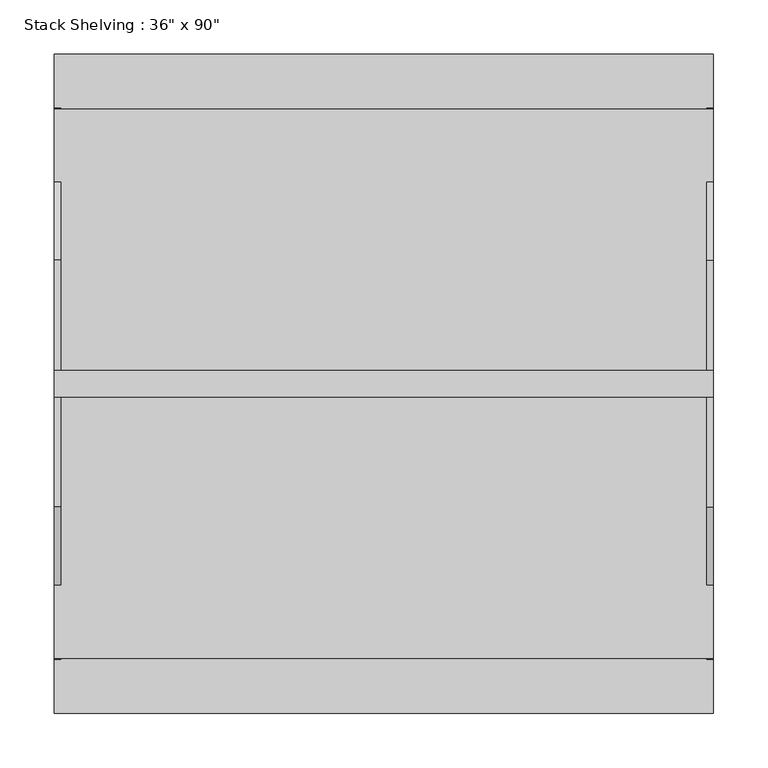
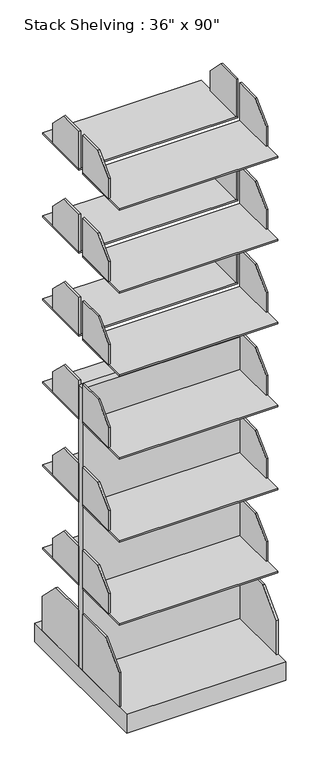
"""IFC4 building model written with IfcOpenShell, lengths in millimetres: proxy geometry."""

from ifc_helpers import new_model, si_unit, frame, origin, origin_with_axes, place, context, project, spatial, polyline, outline, extrude, source, transform, mapped, element, save


def proxy_279d5ef4(model_context):
    return source(origin(), model_context, "Body", "SweptSolid", [
        extrude(outline(polyline([(12.7, 2247.9), (114.3, 2247.9), (186.142049, 2176.057951), (186.142049, 2095.5), (12.7, 2095.5), (12.7, 2247.9)])), frame((-304.8, 0.0, 0.0), z_axis=(1.0, 0.0, 0.0), x_axis=(0.0, 1.0, 0.0)), (0.0, 0.0, 1.0), 6.35),
        extrude(outline(polyline([(165.1, 304.8), (254.9025612, 214.9974388), (254.9025612, 76.2), (12.7, 76.2), (12.7, 304.8), (165.1, 304.8)])), frame((-304.8, 0.0, 0.0), z_axis=(1.0, 0.0, 0.0), x_axis=(0.0, 1.0, 0.0)), (0.0, 0.0, 1.0), 6.35),
        extrude(outline(polyline([(12.7, 1911.35), (114.3, 1911.35), (186.142049, 1839.507951), (186.142049, 1758.95), (12.7, 1758.95), (12.7, 1911.35)])), frame((-304.8, 0.0, 0.0), z_axis=(1.0, 0.0, 0.0), x_axis=(0.0, 1.0, 0.0)), (0.0, 0.0, 1.0), 6.35),
        extrude(outline(polyline([(12.8886472, 1574.8), (114.4886472, 1574.8), (186.3306961, 1502.957951), (186.3306961, 1422.4), (12.8886472, 1422.4), (12.8886472, 1574.8)])), frame((-304.8, 0.0, 0.0), z_axis=(1.0, 0.0, 0.0), x_axis=(0.0, 1.0, 0.0)), (0.0, 0.0, 1.0), 6.35),
        extrude(outline(polyline([(12.8886472, 1238.25), (114.4886472, 1238.25), (186.3306961, 1166.407951), (186.3306961, 1085.85), (12.8886472, 1085.85), (12.8886472, 1238.25)])), frame((-304.8, 0.0, 0.0), z_axis=(1.0, 0.0, 0.0), x_axis=(0.0, 1.0, 0.0)), (0.0, 0.0, 1.0), 6.35),
        extrude(outline(polyline([(12.7, 901.7), (114.3, 901.7), (186.142049, 829.857951), (186.142049, 749.3), (12.7, 749.3), (12.7, 901.7)])), frame((-304.8, 0.0, 0.0), z_axis=(1.0, 0.0, 0.0), x_axis=(0.0, 1.0, 0.0)), (0.0, 0.0, 1.0), 6.35),
        extrude(outline(polyline([(12.7, 565.15), (114.3, 565.15), (186.142049, 493.307951), (186.142049, 412.75), (12.7, 412.75), (12.7, 565.15)])), frame((-304.8, 0.0, 0.0), z_axis=(1.0, 0.0, 0.0), x_axis=(0.0, 1.0, 0.0)), (0.0, 0.0, 1.0), 6.35),
        extrude(outline(polyline([(-12.7, 2247.9), (-12.7, 2095.5), (-186.142049, 2095.5), (-186.142049, 2176.057951), (-114.3, 2247.9), (-12.7, 2247.9)])), frame((-304.8, 0.0, 0.0), z_axis=(1.0, 0.0, 0.0), x_axis=(0.0, 1.0, 0.0)), (0.0, 0.0, 1.0), 6.35),
        extrude(outline(polyline([(-165.1, 304.8), (-12.7, 304.8), (-12.7, 76.2), (-254.9025612, 76.2), (-254.9025612, 214.9974388), (-165.1, 304.8)])), frame((-304.8, 0.0, 0.0), z_axis=(1.0, 0.0, 0.0), x_axis=(0.0, 1.0, 0.0)), (0.0, 0.0, 1.0), 6.35),
        extrude(outline(polyline([(-12.7, 1911.35), (-12.7, 1758.95), (-186.142049, 1758.95), (-186.142049, 1839.507951), (-114.3, 1911.35), (-12.7, 1911.35)])), frame((-304.8, 0.0, 0.0), z_axis=(1.0, 0.0, 0.0), x_axis=(0.0, 1.0, 0.0)), (0.0, 0.0, 1.0), 6.35),
        extrude(outline(polyline([(-12.8886472, 1574.8), (-12.8886472, 1422.4), (-186.3306961, 1422.4), (-186.3306961, 1502.957951), (-114.4886472, 1574.8), (-12.8886472, 1574.8)])), frame((-304.8, 0.0, 0.0), z_axis=(1.0, 0.0, 0.0), x_axis=(0.0, 1.0, 0.0)), (0.0, 0.0, 1.0), 6.35),
        extrude(outline(polyline([(-12.8886472, 1238.25), (-12.8886472, 1085.85), (-186.3306961, 1085.85), (-186.3306961, 1166.407951), (-114.4886472, 1238.25), (-12.8886472, 1238.25)])), frame((-304.8, 0.0, 0.0), z_axis=(1.0, 0.0, 0.0), x_axis=(0.0, 1.0, 0.0)), (0.0, 0.0, 1.0), 6.35),
        extrude(outline(polyline([(-12.7, 901.7), (-12.7, 749.3), (-186.142049, 749.3), (-186.142049, 829.857951), (-114.3, 901.7), (-12.7, 901.7)])), frame((-304.8, 0.0, 0.0), z_axis=(1.0, 0.0, 0.0), x_axis=(0.0, 1.0, 0.0)), (0.0, 0.0, 1.0), 6.35),
        extrude(outline(polyline([(-12.7, 565.15), (-12.7, 412.75), (-186.142049, 412.75), (-186.142049, 493.307951), (-114.3, 565.15), (-12.7, 565.15)])), frame((-304.8, 0.0, 0.0), z_axis=(1.0, 0.0, 0.0), x_axis=(0.0, 1.0, 0.0)), (0.0, 0.0, 1.0), 6.35),
        extrude(outline(polyline([(-12.7, 304.8), (-12.7, 76.2), (-254.9025612, 76.2), (-254.9025612, 214.9974388), (-165.1, 304.8), (-12.7, 304.8)])), frame((298.45, 0.0, 0.0), z_axis=(1.0, 0.0, 0.0), x_axis=(0.0, 1.0, 0.0)), (0.0, 0.0, 1.0), 6.35),
        extrude(outline(polyline([(12.7, 304.8), (165.1, 304.8), (254.9025612, 214.9974388), (254.9025612, 76.2), (12.7, 76.2), (12.7, 304.8)])), frame((298.45, 0.0, 0.0), z_axis=(1.0, 0.0, 0.0), x_axis=(0.0, 1.0, 0.0)), (0.0, 0.0, 1.0), 6.35),
        extrude(outline(polyline([(-12.7, 565.15), (-12.7, 412.75), (-186.142049, 412.75), (-186.142049, 493.307951), (-114.3, 565.15), (-12.7, 565.15)])), frame((298.45, 0.0, 0.0), z_axis=(1.0, 0.0, 0.0), x_axis=(0.0, 1.0, 0.0)), (0.0, 0.0, 1.0), 6.35),
        extrude(outline(polyline([(-12.7, 901.7), (-12.7, 749.3), (-186.142049, 749.3), (-186.142049, 829.857951), (-114.3, 901.7), (-12.7, 901.7)])), frame((298.45, 0.0, 0.0), z_axis=(1.0, 0.0, 0.0), x_axis=(0.0, 1.0, 0.0)), (0.0, 0.0, 1.0), 6.35),
        extrude(outline(polyline([(-12.7, 1238.25), (-12.7, 1085.85), (-186.142049, 1085.85), (-186.142049, 1166.407951), (-114.3, 1238.25), (-12.7, 1238.25)])), frame((298.45, 0.0, 0.0), z_axis=(1.0, 0.0, 0.0), x_axis=(0.0, 1.0, 0.0)), (0.0, 0.0, 1.0), 6.35),
        extrude(outline(polyline([(-12.7, 1574.8), (-12.7, 1422.4), (-186.142049, 1422.4), (-186.142049, 1502.957951), (-114.3, 1574.8), (-12.7, 1574.8)])), frame((298.45, 0.0, 0.0), z_axis=(1.0, 0.0, 0.0), x_axis=(0.0, 1.0, 0.0)), (0.0, 0.0, 1.0), 6.35),
        extrude(outline(polyline([(-12.7, 1911.35), (-12.7, 1758.95), (-186.142049, 1758.95), (-186.142049, 1839.507951), (-114.3, 1911.35), (-12.7, 1911.35)])), frame((298.45, 0.0, 0.0), z_axis=(1.0, 0.0, 0.0), x_axis=(0.0, 1.0, 0.0)), (0.0, 0.0, 1.0), 6.35),
        extrude(outline(polyline([(-12.7, 2247.9), (-12.7, 2095.5), (-186.142049, 2095.5), (-186.142049, 2176.057951), (-114.3, 2247.9), (-12.7, 2247.9)])), frame((298.45, 0.0, 0.0), z_axis=(1.0, 0.0, 0.0), x_axis=(0.0, 1.0, 0.0)), (0.0, 0.0, 1.0), 6.35),
        extrude(outline(polyline([(12.7, 565.15), (114.3, 565.15), (186.142049, 493.307951), (186.142049, 412.75), (12.7, 412.75), (12.7, 565.15)])), frame((298.45, 0.0, 0.0), z_axis=(1.0, 0.0, 0.0), x_axis=(0.0, 1.0, 0.0)), (0.0, 0.0, 1.0), 6.35),
        extrude(outline(polyline([(12.7, 901.7), (114.3, 901.7), (186.142049, 829.857951), (186.142049, 749.3), (12.7, 749.3), (12.7, 901.7)])), frame((298.45, 0.0, 0.0), z_axis=(1.0, 0.0, 0.0), x_axis=(0.0, 1.0, 0.0)), (0.0, 0.0, 1.0), 6.35),
        extrude(outline(polyline([(12.7, 1238.25), (114.3, 1238.25), (186.142049, 1166.407951), (186.142049, 1085.85), (12.7, 1085.85), (12.7, 1238.25)])), frame((298.45, 0.0, 0.0), z_axis=(1.0, 0.0, 0.0), x_axis=(0.0, 1.0, 0.0)), (0.0, 0.0, 1.0), 6.35),
        extrude(outline(polyline([(12.7, 1574.8), (114.3, 1574.8), (186.142049, 1502.957951), (186.142049, 1422.4), (12.7, 1422.4), (12.7, 1574.8)])), frame((298.45, 0.0, 0.0), z_axis=(1.0, 0.0, 0.0), x_axis=(0.0, 1.0, 0.0)), (0.0, 0.0, 1.0), 6.35),
        extrude(outline(polyline([(12.7, 1911.35), (114.3, 1911.35), (186.142049, 1839.507951), (186.142049, 1758.95), (12.7, 1758.95), (12.7, 1911.35)])), frame((298.45, 0.0, 0.0), z_axis=(1.0, 0.0, 0.0), x_axis=(0.0, 1.0, 0.0)), (0.0, 0.0, 1.0), 6.35),
        extrude(outline(polyline([(12.7, 2247.9), (114.3, 2247.9), (186.142049, 2176.057951), (186.142049, 2095.5), (12.7, 2095.5), (12.7, 2247.9)])), frame((298.45, 0.0, 0.0), z_axis=(1.0, 0.0, 0.0), x_axis=(0.0, 1.0, 0.0)), (0.0, 0.0, 1.0), 6.35),
        extrude(outline(polyline([(-304.8, 254.0), (304.8, 254.0), (304.8, 12.7), (-304.8, 12.7), (-304.8, 254.0)])), frame((0.0, 0.0, 406.4), z_axis=(0.0, 0.0, 1.0), x_axis=(1.0, 0.0, 0.0)), (0.0, 0.0, 1.0), 6.35),
        extrude(outline(polyline([(-304.8, 254.0), (304.8, 254.0), (304.8, 12.7), (-304.8, 12.7), (-304.8, 254.0)])), frame((0.0, 0.0, 742.95), z_axis=(0.0, 0.0, 1.0), x_axis=(1.0, 0.0, 0.0)), (0.0, 0.0, 1.0), 6.35),
        extrude(outline(polyline([(-304.8, 254.0), (304.8, 254.0), (304.8, 12.7), (-304.8, 12.7), (-304.8, 254.0)])), frame((0.0, 0.0, 1079.5), z_axis=(0.0, 0.0, 1.0), x_axis=(1.0, 0.0, 0.0)), (0.0, 0.0, 1.0), 6.35),
        extrude(outline(polyline([(-304.8, 254.0), (304.8, 254.0), (304.8, 12.7), (-304.8, 12.7), (-304.8, 254.0)])), frame((0.0, 0.0, 1416.05), z_axis=(0.0, 0.0, 1.0), x_axis=(1.0, 0.0, 0.0)), (0.0, 0.0, 1.0), 6.35),
        extrude(outline(polyline([(-304.8, 254.0), (304.8, 254.0), (304.8, 12.7), (-304.8, 12.7), (-304.8, 254.0)])), frame((0.0, 0.0, 1752.6), z_axis=(0.0, 0.0, 1.0), x_axis=(1.0, 0.0, 0.0)), (0.0, 0.0, 1.0), 6.35),
        extrude(outline(polyline([(-304.8, 254.0), (304.8, 254.0), (304.8, 12.7), (-304.8, 12.7), (-304.8, 254.0)])), frame((0.0, 0.0, 2089.15), z_axis=(0.0, 0.0, 1.0), x_axis=(1.0, 0.0, 0.0)), (0.0, 0.0, 1.0), 6.35),
        extrude(outline(polyline([(304.8, -254.0), (-304.8, -254.0), (-304.8, -12.7), (304.8, -12.7), (304.8, -254.0)])), frame((0.0, 0.0, 406.4), z_axis=(0.0, 0.0, 1.0), x_axis=(1.0, 0.0, 0.0)), (0.0, 0.0, 1.0), 6.35),
        extrude(outline(polyline([(304.8, -254.0), (-304.8, -254.0), (-304.8, -12.7), (304.8, -12.7), (304.8, -254.0)])), frame((0.0, 0.0, 742.95), z_axis=(0.0, 0.0, 1.0), x_axis=(1.0, 0.0, 0.0)), (0.0, 0.0, 1.0), 6.35),
        extrude(outline(polyline([(304.8, -254.0), (-304.8, -254.0), (-304.8, -12.7), (304.8, -12.7), (304.8, -254.0)])), frame((0.0, 0.0, 1079.5), z_axis=(0.0, 0.0, 1.0), x_axis=(1.0, 0.0, 0.0)), (0.0, 0.0, 1.0), 6.35),
        extrude(outline(polyline([(304.8, -254.0), (-304.8, -254.0), (-304.8, -12.7), (304.8, -12.7), (304.8, -254.0)])), frame((0.0, 0.0, 1416.05), z_axis=(0.0, 0.0, 1.0), x_axis=(1.0, 0.0, 0.0)), (0.0, 0.0, 1.0), 6.35),
        extrude(outline(polyline([(304.8, -254.0), (-304.8, -254.0), (-304.8, -12.7), (304.8, -12.7), (304.8, -254.0)])), frame((0.0, 0.0, 1752.6), z_axis=(0.0, 0.0, 1.0), x_axis=(1.0, 0.0, 0.0)), (0.0, 0.0, 1.0), 6.35),
        extrude(outline(polyline([(304.8, -254.0), (-304.8, -254.0), (-304.8, -12.7), (304.8, -12.7), (304.8, -254.0)])), frame((0.0, 0.0, 2089.15), z_axis=(0.0, 0.0, 1.0), x_axis=(1.0, 0.0, 0.0)), (0.0, 0.0, 1.0), 6.35),
        extrude(outline(polyline([(304.8, 12.7), (304.8, -12.7), (-304.8, -12.7), (-304.8, 12.7), (304.8, 12.7)])), frame((0.0, 0.0, 76.2), z_axis=(0.0, 0.0, 1.0), x_axis=(1.0, 0.0, 0.0)), (0.0, 0.0, 1.0), 1143.0),
        extrude(outline(polyline([(304.8, 304.8), (304.8, -304.8), (-304.8, -304.8), (-304.8, 304.8), (304.8, 304.8)])), origin_with_axes(), (0.0, 0.0, 1.0), 76.2),
    ])


if __name__ == "__main__":
    model = new_model("IFC4")
    model_context = context("Model", 3, world=origin())
    ifc_project = project(units=[si_unit("LENGTHUNIT", "METRE", prefix="MILLI")], contexts=[model_context])
    site = spatial("IfcSite", under=ifc_project)
    building = spatial("IfcBuilding", under=site)
    placement = place(None, origin())
    proxy_shape = proxy_279d5ef4(model_context)
    element("IfcBuildingElementProxy", 1, Name="Stack Shelving : 36\" x 90\"", ObjectType="Stack Shelving : 36\" x 90\"", at=placement, inside=building, context=model_context, shape_type="MappedRepresentation", body=[
        mapped(proxy_shape, transform((0.0, 0.0, 0.0), x_axis=(1.0, 0.0, 0.0), y_axis=(0.0, 1.0, 0.0), z_axis=(0.0, 0.0, 1.0))),
    ])
    save(model, "model.ifc")

# Revit data of these elements
# Type "Stack Shelving : 36\" x 90\""
#   Assembly Code = "E1020200"
#   Height = 4' - 0"
#   Width = 2' - 0"
#   Shelving Material = Steel, Paint Finish, Ivory, Glossy
#   Default Elevation = 0
# Element 1 (IfcBuildingElementProxy, "Stack Shelving : 36\" x 90\"")
#   Materials on its faces: "Steel, Paint Finish, Ivory, Glossy"
# Materials
#   "Steel, Paint Finish, Ivory, Glossy": class "Metal", colour RGB 247 247 239, transparency 0, Description = "Steel, paint finish, ivory, glossy", Cost = 0
